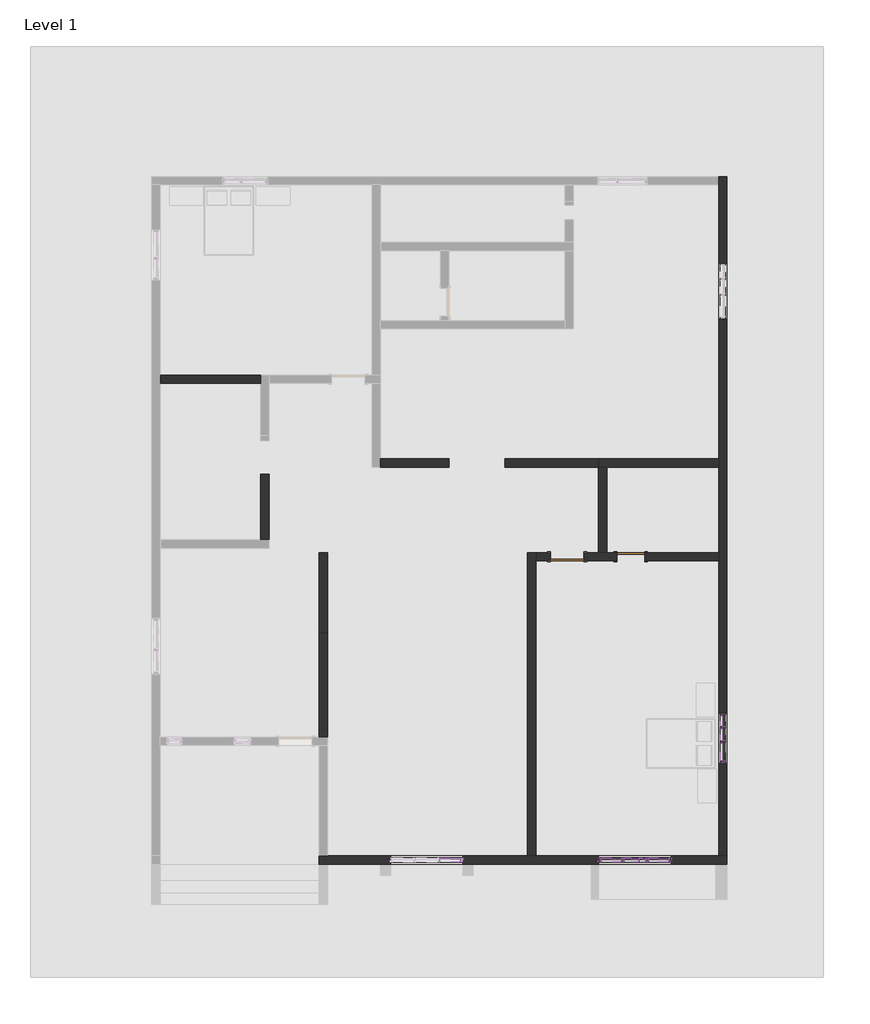
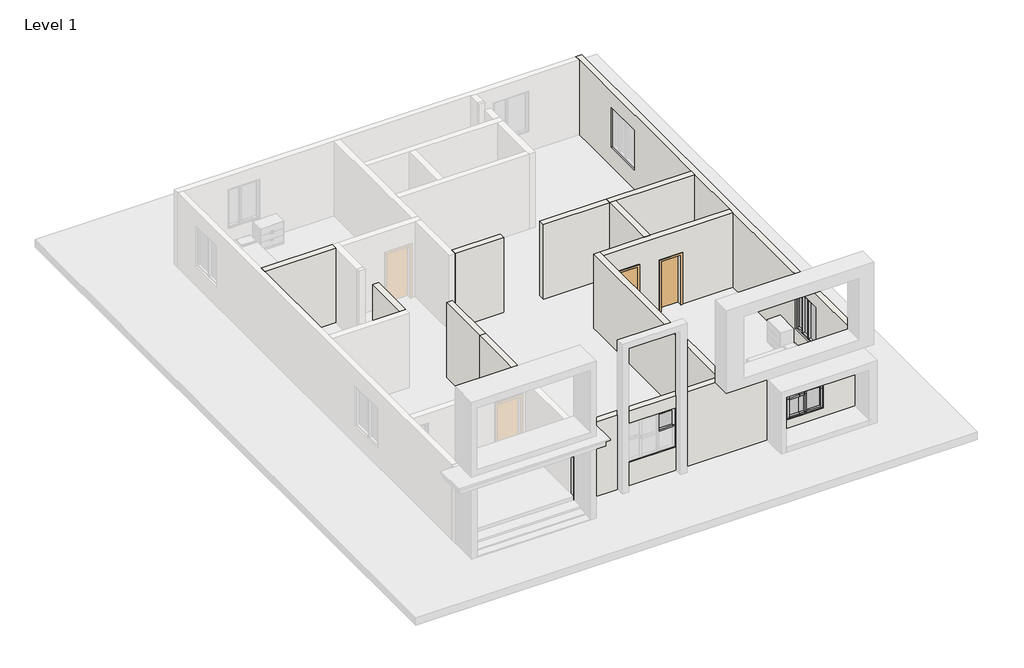
# One storey, part 2 of 3: 40 members, 12 walls, 11 plates, 2 doors.
"""IFC4 building model written with IfcOpenShell, lengths in millimetres."""

from ifc_helpers import new_model, si_unit, origin, origin_with_axes, place, context, project, spatial, polyline, outline, extrude, faceted_brep, transform, mapped, element, save
from components import door_a1484949, door_0ca8825f, member_ff9f2d30, member_6f432376, member_6103f85b, member_495a21e7, member_429f6687, member_fa619fab, member_909e4c35, member_0492494d, member_510dacbd, member_6b3b9dad, member_4557678a, member_702056ca, member_18a184ad, member_34b92440, member_95f02488, member_18dfdc07, member_b9f3750b, member_8199a1f0, member_8c071503, member_78adf786, system_panel_glazed_31c741ab, system_panel_glazed_08392cf6, system_panel_glazed_748c8dd9, system_panel_glazed_a609a774, system_panel_glazed_a541dcfe, system_panel_glazed_71f4521f, system_panel_glazed_f743f071, system_panel_glazed_b692d746, system_panel_glazed_93f5a346, system_panel_glazed_4e9385f6, system_panel_glazed_52ab50c3

model = new_model("IFC4")

# Units and contexts
model_context = context("Model", 3, world=origin())
ifc_project = project(units=[si_unit("LENGTHUNIT", "METRE", prefix="MILLI")], contexts=[model_context])

# Site, building, storey
site = spatial("IfcSite", under=ifc_project)
building = spatial("IfcBuilding", under=site)
storey = spatial("IfcBuildingStorey", under=building, Name="Level 1", Elevation=0.0)

# Doors
placement = place(None, origin())
door_shape = door_a1484949(model_context)
element("IfcDoor", 1, ObjectType="Single-Flush : 30\" x 80\"", at=placement, inside=storey, context=model_context, shape_type="MappedRepresentation", body=[
    mapped(door_shape, transform((-6017.4702714, -3205.7383903, 0.0), x_axis=(1.0, 0.0, 0.0), y_axis=(0.0, 1.0, 0.0), z_axis=(0.0, 0.0, 1.0))),
])
door_2_shape = door_0ca8825f(model_context)
element("IfcDoor", 2, ObjectType="Single-Flush : 36\" x 84\"", at=placement, inside=storey, context=model_context, shape_type="MappedRepresentation", body=[
    mapped(door_2_shape, transform((-7751.0202714, -3205.7383903, 0.0), x_axis=(-1.0, 0.0, 0.0), y_axis=(0.0, -1.0, 0.0), z_axis=(0.0, 0.0, 1.0))),
])

# Members
member_shape = member_ff9f2d30(model_context)
element("IfcMember", 3, ObjectType="Rectangular Mullion : 2.5\" x 5\" rectangular", at=placement, inside=storey, context=model_context, shape_type="MappedRepresentation", body=[
    mapped(member_shape, transform((-3502.8702714, -8228.5883903, 2527.6003844), x_axis=(0.0, 0.0, 1.0), y_axis=(-1.0, 0.0, 0.0), z_axis=(0.0, -1.0, 0.0))),
])
element("IfcMember", 4, ObjectType="Rectangular Mullion : 2.5\" x 5\" rectangular", at=placement, inside=storey, context=model_context, shape_type="MappedRepresentation", body=[
    mapped(member_shape, transform((-3502.8702714, -7898.3883903, 846.465446), x_axis=(0.0, 0.0, -1.0), y_axis=(-1.0, 0.0, 0.0), z_axis=(0.0, 1.0, 0.0))),
])
member_2_shape = member_6f432376(model_context)
element("IfcMember", 5, ObjectType="Rectangular Mullion : 2.5\" x 5\" rectangular", at=placement, inside=storey, context=model_context, shape_type="MappedRepresentation", body=[
    mapped(member_2_shape, transform((-6265.1202714, -11473.4383903, 2256.6794412), x_axis=(0.0, 0.0, 1.0), y_axis=(0.0, -1.0, 0.0), z_axis=(1.0, 0.0, 0.0))),
])
element("IfcMember", 6, ObjectType="Rectangular Mullion : 2.5\" x 5\" rectangular", at=placement, inside=storey, context=model_context, shape_type="MappedRepresentation", body=[
    mapped(member_2_shape, transform((-4976.0702714, -11473.4383903, 2256.6794412), x_axis=(0.0, 0.0, 1.0), y_axis=(0.0, -1.0, 0.0), z_axis=(1.0, 0.0, 0.0))),
])
element("IfcMember", 7, ObjectType="Rectangular Mullion : 2.5\" x 5\" rectangular", at=placement, inside=storey, context=model_context, shape_type="MappedRepresentation", body=[
    mapped(member_2_shape, transform((-5541.2202714, -11473.4383903, 550.0635959), x_axis=(0.0, 0.0, -1.0), y_axis=(0.0, -1.0, 0.0), z_axis=(-1.0, 0.0, 0.0))),
])
element("IfcMember", 8, ObjectType="Rectangular Mullion : 2.5\" x 5\" rectangular", at=placement, inside=storey, context=model_context, shape_type="MappedRepresentation", body=[
    mapped(member_2_shape, transform((-6830.2702714, -11473.4383903, 550.0635959), x_axis=(0.0, 0.0, -1.0), y_axis=(0.0, -1.0, 0.0), z_axis=(-1.0, 0.0, 0.0))),
])
member_3_shape = member_6103f85b(model_context)
element("IfcMember", 9, ObjectType="Rectangular Mullion : 2.5\" x 5\" rectangular", at=placement, inside=storey, context=model_context, shape_type="MappedRepresentation", body=[
    mapped(member_3_shape, transform((-10652.9702714, -11473.4383903, 1807.7366593), x_axis=(0.0, 0.0, 1.0), y_axis=(0.0, -1.0, 0.0), z_axis=(1.0, 0.0, 0.0))),
])
element("IfcMember", 10, ObjectType="Rectangular Mullion : 2.5\" x 5\" rectangular", at=placement, inside=storey, context=model_context, shape_type="MappedRepresentation", body=[
    mapped(member_3_shape, transform((-6265.1202714, -11473.4383903, 1515.2635959), x_axis=(0.0, 0.0, 1.0), y_axis=(0.0, -1.0, 0.0), z_axis=(1.0, 0.0, 0.0))),
])
element("IfcMember", 11, ObjectType="Rectangular Mullion : 2.5\" x 5\" rectangular", at=placement, inside=storey, context=model_context, shape_type="MappedRepresentation", body=[
    mapped(member_3_shape, transform((-4976.0702714, -11473.4383903, 1455.9969292), x_axis=(0.0, 0.0, 1.0), y_axis=(0.0, -1.0, 0.0), z_axis=(1.0, 0.0, 0.0))),
])
member_4_shape = member_495a21e7(model_context)
element("IfcMember", 12, ObjectType="Rectangular Mullion : 2.5\" x 5\" rectangular", at=placement, inside=storey, context=model_context, shape_type="MappedRepresentation", body=[
    mapped(member_4_shape, transform((-10589.4702714, -11473.4383903, 1807.7366593), x_axis=(1.0, 0.0, 0.0), y_axis=(0.0, -1.0, 0.0), z_axis=(0.0, 0.0, -1.0))),
])
member_5_shape = member_429f6687(model_context)
element("IfcMember", 13, ObjectType="Rectangular Mullion : 2.5\" x 5\" rectangular", at=placement, inside=storey, context=model_context, shape_type="MappedRepresentation", body=[
    mapped(member_5_shape, transform((-4912.5702714, -11473.4383903, 550.0635959), x_axis=(1.0, 0.0, 0.0), y_axis=(0.0, -1.0, 0.0), z_axis=(0.0, 0.0, -1.0))),
])
element("IfcMember", 14, ObjectType="Rectangular Mullion : 2.5\" x 5\" rectangular", at=placement, inside=storey, context=model_context, shape_type="MappedRepresentation", body=[
    mapped(member_5_shape, transform((-6893.7702714, -11473.4383903, 1337.4635959), x_axis=(-1.0, 0.0, 0.0), y_axis=(0.0, -1.0, 0.0), z_axis=(0.0, 0.0, 1.0))),
])
member_6_shape = member_fa619fab(model_context)
element("IfcMember", 15, ObjectType="Rectangular Mullion : 2.5\" x 5\" rectangular", at=placement, inside=storey, context=model_context, shape_type="MappedRepresentation", body=[
    mapped(member_6_shape, transform((-5604.7202714, -11473.4383903, 2256.6794412), x_axis=(0.0, 0.0, 1.0), y_axis=(0.0, -1.0, 0.0), z_axis=(1.0, 0.0, 0.0))),
])
member_7_shape = member_909e4c35(model_context)
element("IfcMember", 16, ObjectType="Rectangular Mullion : 2.5\" x 5\" rectangular", at=placement, inside=storey, context=model_context, shape_type="MappedRepresentation", body=[
    mapped(member_7_shape, transform((-6201.6202714, -11473.4383903, 550.0635959), x_axis=(0.0, 0.0, -1.0), y_axis=(0.0, -1.0, 0.0), z_axis=(-1.0, 0.0, 0.0))),
])
element("IfcMember", 17, ObjectType="Rectangular Mullion : 2.5\" x 5\" rectangular", at=placement, inside=storey, context=model_context, shape_type="MappedRepresentation", body=[
    mapped(member_7_shape, transform((-5793.1036047, -11473.4383903, 2256.6794412), x_axis=(0.0, 0.0, 1.0), y_axis=(0.0, -1.0, 0.0), z_axis=(1.0, 0.0, 0.0))),
])
element("IfcMember", 18, ObjectType="Rectangular Mullion : 2.5\" x 5\" rectangular", at=placement, inside=storey, context=model_context, shape_type="MappedRepresentation", body=[
    mapped(member_6_shape, transform((-5793.1036047, -11473.4383903, 550.0635959), x_axis=(0.0, 0.0, -1.0), y_axis=(0.0, -1.0, 0.0), z_axis=(-1.0, 0.0, 0.0))),
])
member_8_shape = member_0492494d(model_context)
element("IfcMember", 19, ObjectType="Rectangular Mullion : 2.5\" x 5\" rectangular", at=placement, inside=storey, context=model_context, shape_type="MappedRepresentation", body=[
    mapped(member_8_shape, transform((-5572.9702714, -11473.4383903, 1515.2635959), x_axis=(1.0, 0.0, 0.0), y_axis=(0.0, -1.0, 0.0), z_axis=(0.0, 0.0, -1.0))),
])
member_9_shape = member_510dacbd(model_context)
element("IfcMember", 20, ObjectType="Rectangular Mullion : 2.5\" x 5\" rectangular", at=placement, inside=storey, context=model_context, shape_type="MappedRepresentation", body=[
    mapped(member_9_shape, transform((-4912.5702714, -11473.4383903, 1515.2635959), x_axis=(1.0, 0.0, 0.0), y_axis=(0.0, -1.0, 0.0), z_axis=(0.0, 0.0, -1.0))),
])
member_10_shape = member_6b3b9dad(model_context)
element("IfcMember", 21, ObjectType="Rectangular Mullion : 2.5\" x 5\" rectangular", at=placement, inside=storey, context=model_context, shape_type="MappedRepresentation", body=[
    mapped(member_10_shape, transform((-6893.7702714, -11473.4383903, 1455.9969292), x_axis=(-1.0, 0.0, 0.0), y_axis=(0.0, -1.0, 0.0), z_axis=(0.0, 0.0, 1.0))),
])
element("IfcMember", 22, ObjectType="Rectangular Mullion : 2.5\" x 5\" rectangular", at=placement, inside=storey, context=model_context, shape_type="MappedRepresentation", body=[
    mapped(member_8_shape, transform((-6233.3702714, -11473.4383903, 1515.2635959), x_axis=(1.0, 0.0, 0.0), y_axis=(0.0, -1.0, 0.0), z_axis=(0.0, 0.0, -1.0))),
])
member_11_shape = member_4557678a(model_context)
element("IfcMember", 23, ObjectType="Rectangular Mullion : 2.5\" x 5\" rectangular", at=placement, inside=storey, context=model_context, shape_type="MappedRepresentation", body=[
    mapped(member_11_shape, transform((-6233.3702714, -11473.4383903, 1455.9969292), x_axis=(1.0, 0.0, 0.0), y_axis=(0.0, -1.0, 0.0), z_axis=(0.0, 0.0, -1.0))),
])
element("IfcMember", 24, ObjectType="Rectangular Mullion : 2.5\" x 5\" rectangular", at=placement, inside=storey, context=model_context, shape_type="MappedRepresentation", body=[
    mapped(member_9_shape, transform((-6893.7702714, -11473.4383903, 2256.6794412), x_axis=(-1.0, 0.0, 0.0), y_axis=(0.0, -1.0, 0.0), z_axis=(0.0, 0.0, 1.0))),
])
member_12_shape = member_702056ca(model_context)
element("IfcMember", 25, ObjectType="Rectangular Mullion : 2.5\" x 5\" rectangular", at=placement, inside=storey, context=model_context, shape_type="MappedRepresentation", body=[
    mapped(member_12_shape, transform((-6893.7702714, -11473.4383903, 1515.2635959), x_axis=(-1.0, 0.0, 0.0), y_axis=(0.0, -1.0, 0.0), z_axis=(0.0, 0.0, 1.0))),
])
member_13_shape = member_18a184ad(model_context)
element("IfcMember", 26, ObjectType="Rectangular Mullion : 2.5\" x 5\" rectangular", at=placement, inside=storey, context=model_context, shape_type="MappedRepresentation", body=[
    mapped(member_13_shape, transform((-6233.3702714, -11473.4383903, 550.0635959), x_axis=(1.0, 0.0, 0.0), y_axis=(0.0, -1.0, 0.0), z_axis=(0.0, 0.0, -1.0))),
])
element("IfcMember", 27, ObjectType="Rectangular Mullion : 2.5\" x 5\" rectangular", at=placement, inside=storey, context=model_context, shape_type="MappedRepresentation", body=[
    mapped(member_13_shape, transform((-5572.9702714, -11473.4383903, 550.0635959), x_axis=(1.0, 0.0, 0.0), y_axis=(0.0, -1.0, 0.0), z_axis=(0.0, 0.0, -1.0))),
])
member_14_shape = member_34b92440(model_context)
element("IfcMember", 28, ObjectType="Rectangular Mullion : 2.5\" x 5\" rectangular", at=placement, inside=storey, context=model_context, shape_type="MappedRepresentation", body=[
    mapped(member_14_shape, transform((-6233.3702714, -11473.4383903, 1337.4635959), x_axis=(1.0, 0.0, 0.0), y_axis=(0.0, -1.0, 0.0), z_axis=(0.0, 0.0, -1.0))),
])
member_15_shape = member_95f02488(model_context)
element("IfcMember", 29, ObjectType="Rectangular Mullion : 2.5\" x 5\" rectangular", at=placement, inside=storey, context=model_context, shape_type="MappedRepresentation", body=[
    mapped(member_15_shape, transform((-5604.7202714, -11473.4383903, 1337.4635959), x_axis=(0.0, 0.0, 1.0), y_axis=(0.0, -1.0, 0.0), z_axis=(1.0, 0.0, 0.0))),
])
member_16_shape = member_18dfdc07(model_context)
element("IfcMember", 30, ObjectType="Rectangular Mullion : 2.5\" x 5\" rectangular", at=placement, inside=storey, context=model_context, shape_type="MappedRepresentation", body=[
    mapped(member_16_shape, transform((-5793.1036047, -11473.4383903, 1337.4635959), x_axis=(0.0, 0.0, 1.0), y_axis=(0.0, -1.0, 0.0), z_axis=(1.0, 0.0, 0.0))),
])
element("IfcMember", 31, ObjectType="Rectangular Mullion : 2.5\" x 5\" rectangular", at=placement, inside=storey, context=model_context, shape_type="MappedRepresentation", body=[
    mapped(member_14_shape, transform((-5572.9702714, -11473.4383903, 1337.4635959), x_axis=(1.0, 0.0, 0.0), y_axis=(0.0, -1.0, 0.0), z_axis=(0.0, 0.0, -1.0))),
])
element("IfcMember", 32, ObjectType="Rectangular Mullion : 2.5\" x 5\" rectangular", at=placement, inside=storey, context=model_context, shape_type="MappedRepresentation", body=[
    mapped(member_11_shape, transform((-5572.9702714, -11473.4383903, 1455.9969292), x_axis=(1.0, 0.0, 0.0), y_axis=(0.0, -1.0, 0.0), z_axis=(0.0, 0.0, -1.0))),
])
element("IfcMember", 33, ObjectType="Rectangular Mullion : 2.5\" x 5\" rectangular", at=placement, inside=storey, context=model_context, shape_type="MappedRepresentation", body=[
    mapped(member_10_shape, transform((-4912.5702714, -11473.4383903, 1337.4635959), x_axis=(1.0, 0.0, 0.0), y_axis=(0.0, -1.0, 0.0), z_axis=(0.0, 0.0, -1.0))),
])
element("IfcMember", 34, ObjectType="Rectangular Mullion : 2.5\" x 5\" rectangular", at=placement, inside=storey, context=model_context, shape_type="MappedRepresentation", body=[
    mapped(member_12_shape, transform((-4912.5702714, -11473.4383903, 1455.9969292), x_axis=(1.0, 0.0, 0.0), y_axis=(0.0, -1.0, 0.0), z_axis=(0.0, 0.0, -1.0))),
])
member_17_shape = member_b9f3750b(model_context)
element("IfcMember", 35, ObjectType="Rectangular Mullion : 2.5\" x 5\" rectangular", at=placement, inside=storey, context=model_context, shape_type="MappedRepresentation", body=[
    mapped(member_17_shape, transform((-3502.8702714, -8292.0883903, 846.465446), x_axis=(0.0, 0.0, -1.0), y_axis=(-1.0, 0.0, 0.0), z_axis=(0.0, 1.0, 0.0))),
])
member_18_shape = member_8199a1f0(model_context)
element("IfcMember", 36, ObjectType="Rectangular Mullion : 2.5\" x 5\" rectangular", at=placement, inside=storey, context=model_context, shape_type="MappedRepresentation", body=[
    mapped(member_18_shape, transform((-3502.8702714, -7536.4383903, 846.465446), x_axis=(0.0, 0.0, -1.0), y_axis=(-1.0, 0.0, 0.0), z_axis=(0.0, 1.0, 0.0))),
])
member_19_shape = member_8c071503(model_context)
element("IfcMember", 37, ObjectType="Rectangular Mullion : 2.5\" x 5\" rectangular", at=placement, inside=storey, context=model_context, shape_type="MappedRepresentation", body=[
    mapped(member_19_shape, transform((-3502.8702714, -8260.3383903, 846.465446), x_axis=(0.0, -1.0, 0.0), y_axis=(-1.0, 0.0, 0.0), z_axis=(0.0, 0.0, -1.0))),
])
element("IfcMember", 38, ObjectType="Rectangular Mullion : 2.5\" x 5\" rectangular", at=placement, inside=storey, context=model_context, shape_type="MappedRepresentation", body=[
    mapped(member_19_shape, transform((-3502.8702714, -7866.6383903, 846.465446), x_axis=(0.0, -1.0, 0.0), y_axis=(-1.0, 0.0, 0.0), z_axis=(0.0, 0.0, -1.0))),
])
element("IfcMember", 39, ObjectType="Rectangular Mullion : 2.5\" x 5\" rectangular", at=placement, inside=storey, context=model_context, shape_type="MappedRepresentation", body=[
    mapped(member_18_shape, transform((-3502.8702714, -7834.8883903, 2527.6003844), x_axis=(0.0, 0.0, 1.0), y_axis=(-1.0, 0.0, 0.0), z_axis=(0.0, -1.0, 0.0))),
])
element("IfcMember", 40, ObjectType="Rectangular Mullion : 2.5\" x 5\" rectangular", at=placement, inside=storey, context=model_context, shape_type="MappedRepresentation", body=[
    mapped(member_17_shape, transform((-3502.8702714, -8781.0383903, 2527.6003844), x_axis=(0.0, 0.0, 1.0), y_axis=(-1.0, 0.0, 0.0), z_axis=(0.0, -1.0, 0.0))),
])
member_20_shape = member_78adf786(model_context)
element("IfcMember", 41, ObjectType="Rectangular Mullion : 2.5\" x 5\" rectangular", at=placement, inside=storey, context=model_context, shape_type="MappedRepresentation", body=[
    mapped(member_20_shape, transform((-3502.8702714, -7472.9383903, 2527.6003844), x_axis=(0.0, 1.0, 0.0), y_axis=(-1.0, 0.0, 0.0), z_axis=(0.0, 0.0, 1.0))),
])
element("IfcMember", 42, ObjectType="Rectangular Mullion : 2.5\" x 5\" rectangular", at=placement, inside=storey, context=model_context, shape_type="MappedRepresentation", body=[
    mapped(member_20_shape, transform((-3502.8702714, -8844.5383903, 846.465446), x_axis=(0.0, -1.0, 0.0), y_axis=(-1.0, 0.0, 0.0), z_axis=(0.0, 0.0, -1.0))),
])

# Plates
system_panel_glazed_shape = system_panel_glazed_31c741ab(model_context)
element("IfcPlate", 43, ObjectType="System Panel : Glazed", at=placement, inside=storey, context=model_context, shape_type="MappedRepresentation", body=[
    mapped(system_panel_glazed_shape, transform((-10935.5452714, -11473.4383903, 1839.4866593), x_axis=(1.0, 0.0, 0.0), y_axis=(0.0, 1.0, 0.0), z_axis=(0.0, 0.0, 1.0))),
])
system_panel_glazed_2_shape = system_panel_glazed_08392cf6(model_context)
element("IfcPlate", 44, ObjectType="System Panel : Glazed", at=placement, inside=storey, context=model_context, shape_type="MappedRepresentation", body=[
    mapped(system_panel_glazed_2_shape, transform((-6547.6952714, -11473.4383903, 613.5635959), x_axis=(1.0, 0.0, 0.0), y_axis=(0.0, 1.0, 0.0), z_axis=(0.0, 0.0, 1.0))),
])
system_panel_glazed_3_shape = system_panel_glazed_748c8dd9(model_context)
element("IfcPlate", 45, ObjectType="System Panel : Glazed", at=placement, inside=storey, context=model_context, shape_type="MappedRepresentation", body=[
    mapped(system_panel_glazed_3_shape, transform((-6547.6952714, -11473.4383903, 1547.0135959), x_axis=(1.0, 0.0, 0.0), y_axis=(0.0, 1.0, 0.0), z_axis=(0.0, 0.0, 1.0))),
])
system_panel_glazed_4_shape = system_panel_glazed_a609a774(model_context)
element("IfcPlate", 46, ObjectType="System Panel : Glazed", at=placement, inside=storey, context=model_context, shape_type="MappedRepresentation", body=[
    mapped(system_panel_glazed_4_shape, transform((-5997.3619381, -11473.4383903, 613.5635959), x_axis=(1.0, 0.0, 0.0), y_axis=(0.0, 1.0, 0.0), z_axis=(0.0, 0.0, 1.0))),
])
system_panel_glazed_5_shape = system_panel_glazed_a541dcfe(model_context)
element("IfcPlate", 47, ObjectType="System Panel : Glazed", at=placement, inside=storey, context=model_context, shape_type="MappedRepresentation", body=[
    mapped(system_panel_glazed_5_shape, transform((-5903.1702714, -11473.4383903, 1369.2135959), x_axis=(1.0, 0.0, 0.0), y_axis=(0.0, 1.0, 0.0), z_axis=(0.0, 0.0, 1.0))),
])
system_panel_glazed_6_shape = system_panel_glazed_71f4521f(model_context)
element("IfcPlate", 48, ObjectType="System Panel : Glazed", at=placement, inside=storey, context=model_context, shape_type="MappedRepresentation", body=[
    mapped(system_panel_glazed_6_shape, transform((-5698.9119381, -11473.4383903, 613.5635959), x_axis=(1.0, 0.0, 0.0), y_axis=(0.0, 1.0, 0.0), z_axis=(0.0, 0.0, 1.0))),
])
system_panel_glazed_7_shape = system_panel_glazed_f743f071(model_context)
element("IfcPlate", 49, ObjectType="System Panel : Glazed", at=placement, inside=storey, context=model_context, shape_type="MappedRepresentation", body=[
    mapped(system_panel_glazed_7_shape, transform((-5258.6452714, -11473.4383903, 613.5635959), x_axis=(1.0, 0.0, 0.0), y_axis=(0.0, 1.0, 0.0), z_axis=(0.0, 0.0, 1.0))),
])
system_panel_glazed_8_shape = system_panel_glazed_b692d746(model_context)
element("IfcPlate", 50, ObjectType="System Panel : Glazed", at=placement, inside=storey, context=model_context, shape_type="MappedRepresentation", body=[
    mapped(system_panel_glazed_8_shape, transform((-5258.6452714, -11473.4383903, 1487.7469292), x_axis=(1.0, 0.0, 0.0), y_axis=(0.0, 1.0, 0.0), z_axis=(0.0, 0.0, 1.0))),
])
system_panel_glazed_9_shape = system_panel_glazed_93f5a346(model_context)
element("IfcPlate", 51, ObjectType="System Panel : Glazed", at=placement, inside=storey, context=model_context, shape_type="MappedRepresentation", body=[
    mapped(system_panel_glazed_9_shape, transform((-3502.8702714, -7685.6633903, 909.965446), x_axis=(0.0, -1.0, 0.0), y_axis=(1.0, 0.0, 0.0), z_axis=(0.0, 0.0, 1.0))),
])
system_panel_glazed_10_shape = system_panel_glazed_4e9385f6(model_context)
element("IfcPlate", 52, ObjectType="System Panel : Glazed", at=placement, inside=storey, context=model_context, shape_type="MappedRepresentation", body=[
    mapped(system_panel_glazed_10_shape, transform((-3502.8702714, -8536.5633903, 909.965446), x_axis=(0.0, -1.0, 0.0), y_axis=(1.0, 0.0, 0.0), z_axis=(0.0, 0.0, 1.0))),
])
system_panel_glazed_11_shape = system_panel_glazed_52ab50c3(model_context)
element("IfcPlate", 53, ObjectType="System Panel : Glazed", at=placement, inside=storey, context=model_context, shape_type="MappedRepresentation", body=[
    mapped(system_panel_glazed_11_shape, transform((-3502.8702714, -8063.4883903, 909.965446), x_axis=(0.0, -1.0, 0.0), y_axis=(1.0, 0.0, 0.0), z_axis=(0.0, 0.0, 1.0))),
])

# Walls
element("IfcWall", 54, ObjectType="9\"", at=placement, inside=storey, context=model_context, shape_type="Brep", body=[
    faceted_brep([(-3388.5702714, -11359.1383903, 0.0), (-3388.5702714, 7157.4616097, 0.0), (-3388.5702714, 7157.4616097, 3048.0), (-3388.5702714, -11359.1383903, 3048.0), (-3388.5702714, -7472.9383903, 2527.6003844), (-3388.5702714, -7472.9383903, 846.465446), (-3388.5702714, -8844.5383903, 846.465446), (-3388.5702714, -8844.5383903, 2527.6003844), (-3388.5702714, 4795.2616097, 2404.522235), (-3388.5702714, 4795.2616097, 784.7381643), (-3388.5702714, 3271.2616097, 784.7381643), (-3388.5702714, 3271.2616097, 2404.522235), (-3617.1702714, 7157.4616097, 0.0), (-3617.1702714, 6928.8616097, 0.0), (-3617.1702714, -538.7383903, 0.0), (-3617.1702714, -767.3383903, 0.0), (-3617.1702714, -3091.4383903, 0.0), (-3617.1702714, -3320.0383903, 0.0), (-3617.1702714, -11359.1383903, 0.0), (-3617.1702714, -11359.1383903, 3048.0), (-3617.1702714, -3320.0383903, 3048.0), (-3617.1702714, -3091.4383903, 3048.0), (-3617.1702714, -767.3383903, 3048.0), (-3617.1702714, -538.7383903, 3048.0), (-3617.1702714, 6928.8616097, 3048.0), (-3617.1702714, 7157.4616097, 3048.0), (-3617.1702714, -7472.9383903, 846.465446), (-3617.1702714, -7472.9383903, 2527.6003844), (-3617.1702714, -8844.5383903, 2527.6003844), (-3617.1702714, -8844.5383903, 846.465446), (-3617.1702714, 4795.2616097, 784.7381643), (-3617.1702714, 4795.2616097, 2404.522235), (-3617.1702714, 3271.2616097, 2404.522235), (-3617.1702714, 3271.2616097, 784.7381643)], [[[0, 1, 2, 3], [4, 5, 6, 7], [8, 9, 10, 11]], [[12, 13, 14, 15, 16, 17, 18, 19, 20, 21, 22, 23, 24, 25], [26, 27, 28, 29], [30, 31, 32, 33]], [[1, 0, 18, 17, 16, 15, 14, 13, 12]], [[3, 2, 25, 24, 23, 22, 21, 20, 19]], [[0, 3, 19, 18]], [[2, 1, 12, 25]], [[4, 27, 26, 5]], [[27, 4, 7, 28]], [[28, 7, 6, 29]], [[5, 26, 29, 6]], [[30, 9, 8, 31]], [[31, 8, 11, 32]], [[32, 11, 10, 33]], [[9, 30, 33, 10]]]),
])
element("IfcWall", 55, ObjectType="9\"", at=placement, inside=storey, context=model_context, shape_type="SweptSolid", body=[
    extrude(outline(polyline([(-14285.1702714, -5294.8883903), (-14285.1702714, -8120.6383903), (-14513.7702714, -8120.6383903), (-14513.7702714, -5294.8883903), (-14285.1702714, -5294.8883903)])), origin_with_axes(), (0.0, 0.0, 1.0), 3048.0),
])
element("IfcWall", 56, ObjectType="9\"", at=placement, inside=storey, context=model_context, shape_type="Brep", body=[
    faceted_brep([(-8608.2702714, -11359.1383903, 0.0), (-8608.2702714, -3320.0383903, 0.0), (-8608.2702714, -3091.4383903, 0.0), (-8608.2702714, -3091.4383903, 3048.0), (-8608.2702714, -3320.0383903, 3048.0), (-8608.2702714, -11359.1383903, 3048.0), (-8836.8702714, -11359.1383903, 0.0), (-8836.8702714, -11359.1383903, 3048.0), (-8836.8702714, -3091.4383903, 3048.0), (-8836.8702714, -3091.4383903, 0.0)], [[[0, 1, 2, 3, 4, 5]], [[6, 7, 8, 9]], [[2, 1, 0, 6, 9]], [[5, 4, 3, 8, 7]], [[0, 5, 7, 6]], [[3, 2, 9, 8]]]),
])
element("IfcWall", 57, ObjectType="9\"", at=placement, inside=storey, context=model_context, shape_type="Brep", body=[
    faceted_brep([(-5636.4702714, -3320.0383903, 2032.0), (-5636.4702714, -3320.0383903, 0.0), (-3617.1702714, -3320.0383903, 0.0), (-3617.1702714, -3320.0383903, 3048.0), (-8608.2702714, -3320.0383903, 3048.0), (-8608.2702714, -3320.0383903, 0.0), (-8208.2202714, -3320.0383903, 0.0), (-8208.2202714, -3320.0383903, 2133.6), (-7293.8202714, -3320.0383903, 2133.6), (-7293.8202714, -3320.0383903, 0.0), (-6398.4702714, -3320.0383903, 0.0), (-6398.4702714, -3320.0383903, 2032.0), (-3617.1702714, -3091.4383903, 0.0), (-5636.4702714, -3091.4383903, 0.0), (-5636.4702714, -3091.4383903, 2032.0), (-6398.4702714, -3091.4383903, 2032.0), (-6398.4702714, -3091.4383903, 0.0), (-6665.1702714, -3091.4383903, 0.0), (-6893.7702714, -3091.4383903, 0.0), (-7293.8202714, -3091.4383903, 0.0), (-7293.8202714, -3091.4383903, 2133.6), (-8208.2202714, -3091.4383903, 2133.6), (-8208.2202714, -3091.4383903, 0.0), (-8608.2702714, -3091.4383903, 0.0), (-8608.2702714, -3091.4383903, 3048.0), (-6893.7702714, -3091.4383903, 3048.0), (-6665.1702714, -3091.4383903, 3048.0), (-3617.1702714, -3091.4383903, 3048.0)], [[[0, 1, 2, 3, 4, 5, 6, 7, 8, 9, 10, 11]], [[12, 13, 14, 15, 16, 17, 18, 19, 20, 21, 22, 23, 24, 25, 26, 27]], [[23, 22, 6, 5]], [[10, 9, 19, 18, 17, 16]], [[2, 1, 13, 12]], [[4, 3, 27, 26, 25, 24]], [[5, 4, 24, 23]], [[3, 2, 12, 27]], [[7, 6, 22, 21]], [[8, 7, 21, 20]], [[9, 8, 20, 19]], [[14, 13, 1, 0]], [[15, 14, 0, 11]], [[16, 15, 11, 10]]]),
])
element("IfcWall", 58, ObjectType="9\"", at=placement, inside=storey, context=model_context, shape_type="Brep", body=[
    faceted_brep([(-3617.1702714, -538.7383903, 0.0), (-6893.7702714, -538.7383903, 0.0), (-6893.7702714, -538.7383903, 3048.0), (-3617.1702714, -538.7383903, 3048.0), (-3617.1702714, -767.3383903, 0.0), (-3617.1702714, -767.3383903, 3048.0), (-6665.1702714, -767.3383903, 3048.0), (-6893.7702714, -767.3383903, 3048.0), (-6893.7702714, -767.3383903, 0.0), (-6665.1702714, -767.3383903, 0.0)], [[[0, 1, 2, 3]], [[4, 5, 6, 7, 8, 9]], [[1, 0, 4, 9, 8]], [[3, 2, 7, 6, 5]], [[0, 3, 5, 4]], [[2, 1, 8, 7]]]),
])
element("IfcWall", 59, ObjectType="9\"", at=placement, inside=storey, context=model_context, shape_type="SweptSolid", body=[
    extrude(outline(polyline([(-6893.7702714, -3091.4383903), (-6893.7702714, -767.3383903), (-6665.1702714, -767.3383903), (-6665.1702714, -3091.4383903), (-6893.7702714, -3091.4383903)])), origin_with_axes(), (0.0, 0.0, 1.0), 3048.0),
])
element("IfcWall", 60, ObjectType="9\"", at=placement, inside=storey, context=model_context, shape_type="SweptSolid", body=[
    extrude(outline(polyline([(-15885.3702714, -957.8383903), (-15885.3702714, -2748.5383903), (-16113.9702714, -2748.5383903), (-16113.9702714, -957.8383903), (-15885.3702714, -957.8383903)])), origin_with_axes(), (0.0, 0.0, 1.0), 3048.0),
])
element("IfcWall", 61, ObjectType="9\"", at=placement, inside=storey, context=model_context, shape_type="SweptSolid", body=[
    extrude(outline(polyline([(-18857.1702714, 1747.2616097), (-16113.9702714, 1747.2616097), (-16113.9702714, 1518.6616097), (-18857.1702714, 1518.6616097), (-18857.1702714, 1747.2616097)])), origin_with_axes(), (0.0, 0.0, 1.0), 3048.0),
])
element("IfcWall", 62, ObjectType="9\"", at=placement, inside=storey, context=model_context, shape_type="SweptSolid", body=[
    extrude(outline(polyline([(-10970.4702714, -767.3383903), (-12837.3702714, -767.3383903), (-12837.3702714, -538.7383903), (-10970.4702714, -538.7383903), (-10970.4702714, -767.3383903)])), origin_with_axes(), (0.0, 0.0, 1.0), 3048.0),
])
element("IfcWall", 63, ObjectType="9\"", at=placement, inside=storey, context=model_context, shape_type="SweptSolid", body=[
    extrude(outline(polyline([(-6893.7702714, -767.3383903), (-9446.4702714, -767.3383903), (-9446.4702714, -538.7383903), (-6893.7702714, -538.7383903), (-6893.7702714, -767.3383903)])), origin_with_axes(), (0.0, 0.0, 1.0), 3048.0),
])
element("IfcWall", 64, ObjectType="9\"", at=placement, inside=storey, context=model_context, shape_type="Brep", body=[
    faceted_brep([(-14513.7702714, -11587.7383903, 0.0), (-3388.5702714, -11587.7383903, 0.0), (-3388.5702714, -11587.7383903, 3048.0), (-14513.7702714, -11587.7383903, 3048.0), (-12570.6702714, -11587.7383903, 948.7091628), (-12570.6702714, -11587.7383903, 2531.2974891), (-10589.4702714, -11587.7383903, 2531.2974891), (-10589.4702714, -11587.7383903, 948.7091628), (-6893.7702714, -11587.7383903, 550.0635959), (-6893.7702714, -11587.7383903, 2256.6794412), (-4912.5702714, -11587.7383903, 2256.6794412), (-4912.5702714, -11587.7383903, 550.0635959), (-3388.5702714, -11359.1383903, 0.0), (-3617.1702714, -11359.1383903, 0.0), (-8608.2702714, -11359.1383903, 0.0), (-8836.8702714, -11359.1383903, 0.0), (-14285.1702714, -11359.1383903, 0.0), (-14513.7702714, -11359.1383903, 0.0), (-14513.7702714, -11359.1383903, 3048.0), (-14285.1702714, -11359.1383903, 3048.0), (-8836.8702714, -11359.1383903, 3048.0), (-8608.2702714, -11359.1383903, 3048.0), (-3617.1702714, -11359.1383903, 3048.0), (-3388.5702714, -11359.1383903, 3048.0), (-12570.6702714, -11359.1383903, 2531.2974891), (-12570.6702714, -11359.1383903, 948.7091628), (-10589.4702714, -11359.1383903, 948.7091628), (-10589.4702714, -11359.1383903, 2531.2974891), (-6893.7702714, -11359.1383903, 2256.6794412), (-6893.7702714, -11359.1383903, 550.0635959), (-4912.5702714, -11359.1383903, 550.0635959), (-4912.5702714, -11359.1383903, 2256.6794412)], [[[0, 1, 2, 3], [4, 5, 6, 7], [8, 9, 10, 11]], [[12, 13, 14, 15, 16, 17, 18, 19, 20, 21, 22, 23], [24, 25, 26, 27], [28, 29, 30, 31]], [[1, 0, 17, 16, 15, 14, 13, 12]], [[3, 2, 23, 22, 21, 20, 19, 18]], [[0, 3, 18, 17]], [[2, 1, 12, 23]], [[24, 5, 4, 25]], [[5, 24, 27, 6]], [[6, 27, 26, 7]], [[25, 4, 7, 26]], [[8, 29, 28, 9]], [[9, 28, 31, 10]], [[10, 31, 30, 11]], [[29, 8, 11, 30]]]),
])
element("IfcWall", 65, ObjectType="9\"", at=placement, inside=storey, context=model_context, shape_type="SweptSolid", body=[
    extrude(outline(polyline([(-14285.1702714, -3091.4383903), (-14285.1702714, -5294.8883903), (-14513.7702714, -5294.8883903), (-14513.7702714, -3091.4383903), (-14285.1702714, -3091.4383903)])), origin_with_axes(), (0.0, 0.0, 1.0), 3048.0),
])

save(model, "model.ifc")

# Revit data of these elements
# Type "Single-Flush : 30\" x 80\""
#   Type Mark = "5"
#   Construction Type Id = "MDOOR"
#   Assembly Code = "C1020"
#   Analytic Construction = "Metal"
#   Thickness = 0' - 2"
#   Heat Transfer Coefficient (U) = 0.651978 BTU/(h·ft²·°F)
#   Height = 6' - 8"
#   Trim Projection Ext = 0' - 1"
#   Trim Projection Int = 0' - 1"
#   Trim Width = 0' - 3"
#   Width = 2' - 6"
#   Define Thermal Properties by = 1
#   Define Thermal Properties by = 1
#   Door Material = Door - Panel
#   Frame Material = Door - Frame
#   Visual Light Transmittance = 0
#   Solar Heat Gain Coefficient = 0
#   Function = (empty or 0)
#   Wall Closure = (empty or 0)
# Type "Single-Flush : 36\" x 84\""
#   Type Mark = "1"
#   Construction Type Id = "MDOOR"
#   Assembly Code = "C1020"
#   Analytic Construction = "Metal"
#   Thickness = 0' - 2"
#   Heat Transfer Coefficient (U) = 0.651978 BTU/(h·ft²·°F)
#   Height = 7' - 0"
#   Trim Projection Ext = 0' - 1"
#   Trim Projection Int = 0' - 1"
#   Trim Width = 0' - 3"
#   Width = 3' - 0"
#   Define Thermal Properties by = 1
#   Define Thermal Properties by = 1
#   Door Material = Door - Panel
#   Frame Material = Door - Frame
#   Visual Light Transmittance = 0
#   Solar Heat Gain Coefficient = 0
#   Function = (empty or 0)
#   Wall Closure = (empty or 0)
# Type "Rectangular Mullion : 2.5\" x 5\" rectangular"
#   built-in parameter 1007304 = 0.416667 (stored number, unit not read)
#   built-in parameter 1007301 = 0.104167 (stored number, unit not read)
#   built-in parameter 1007300 = 0.104167 (stored number, unit not read)
# Type "System Panel : Glazed"
#   Construction Type Id = "GSP4R"
#   Analytic Construction = "1/8 in Pilkington single glazing"
#   Visual Light Transmittance = 0.9
#   Solar Heat Gain Coefficient = 0.86
#   Heat Transfer Coefficient (U) = 1.18115 BTU/(h·ft²·°F)
#   Define Thermal Properties by = 1
# Type "9\""
#   Assembly Code = "B2010"
#   Layers, outside or top first: 0' - 9" no material (function 1)
# Element 1 (IfcDoor, "Single-Flush : 30\" x 80\"")
#   Phase Created = New Construction
#   Materials on its faces: "Door - Frame", "Door - Panel"
# Element 2 (IfcDoor, "Single-Flush : 36\" x 84\"")
#   Phase Created = New Construction
#   Materials on its faces: "Door - Frame", "Door - Panel"
# Elements 3, 4, 5, 6, 7, 8, 9, 10, 11, 12, 13, 14, 15, 16, 17, 18, 19, 20, 21, 22, 23, 24, 25, 26, 27, 28, 29, 30, 31, 32, 33, 34, 35, 36, 37, 38, 39, 40, 41, 42 (IfcMember, "Rectangular Mullion : 2.5\" x 5\" rectangular")
#   Phase Created = New Construction
#   Materials on its faces: "Aluminum"
# Elements 43, 44, 45, 46, 47, 48, 49, 50, 51, 52, 53 (IfcPlate, "System Panel : Glazed")
#   Phase Created = New Construction
#   Materials on its faces: "Glass"
# Elements 54, 55, 56, 57, 58, 59, 60, 61, 62, 63, 64, 65 (IfcWall, "9\"")
#   Top Offset = 0' - 0"
#   Base Offset = 0' - 0"
#   Unconnected Height = 10' - 0"
#   wall height = 10' - 0"
#   Phase Created = New Construction
#   Base Constraint = Level 1
#   Materials on its faces: "Default Wall"
# Materials
#   "Door - Panel": class "Wood", colour RGB 210 159 95, transparency 0, Cost = 0
#   "Door - Frame": colour RGB 118 70 51, transparency 0, Cost = 0
#   "Aluminum": class "Metal", colour RGB 247 247 247, transparency 0, Description = "Aluminum 6061", Cost = 0
#   "Glass": class "Glass", colour RGB 0 128 192, transparency 0.75, Description = "Soda Lime Glass", Cost = 0
#   "Default Wall": colour RGB 128 128 128, transparency 0, Cost = 0
